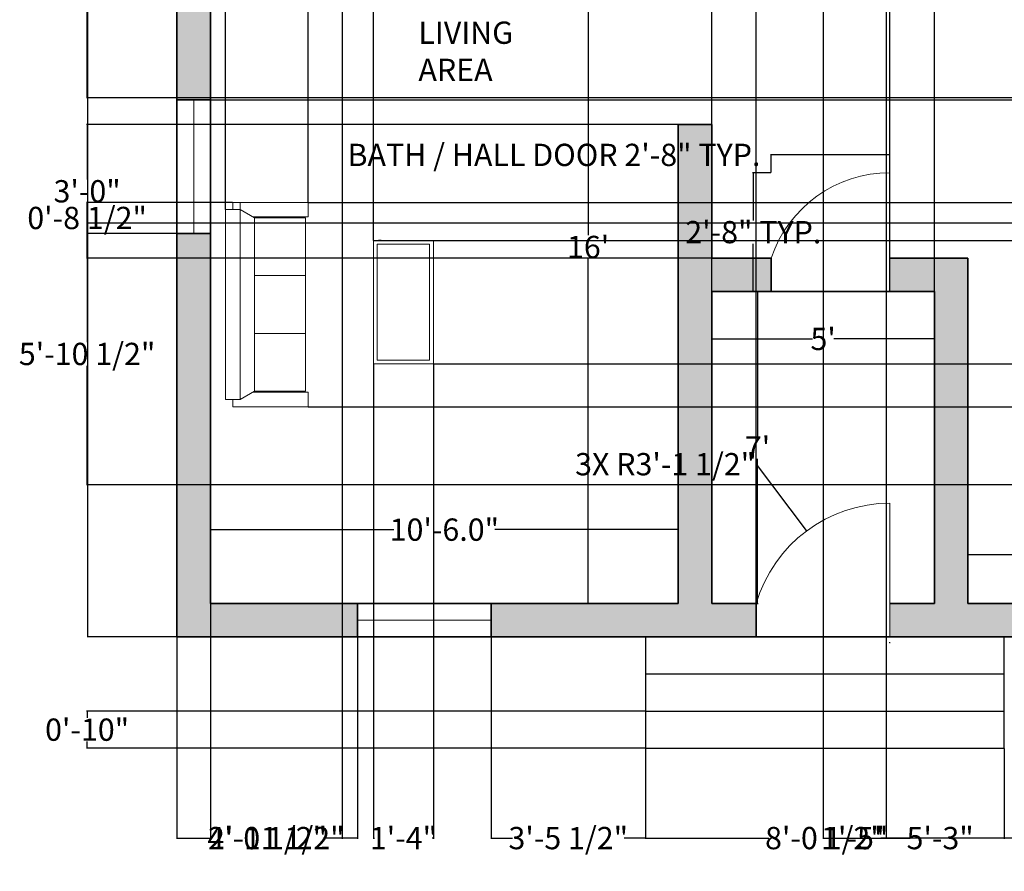
# Model space of a CAD drawing. Units: inches. Extents: x 1174 to 1615, y 3112 to 3628.
# Tile 1 of 6: x 1174 to 1439, y 3112 to 3341. Entities that reach past the tile are written whole.
import ezdxf

# ---------------------------------------------------------------- set-up
doc = ezdxf.new("R2010")
doc.units = ezdxf.units.IN
doc.header["$MEASUREMENT"] = 0
doc.layers.get('0').update_dxf_attribs({"color": 250})
for name, color, linetype, lineweight in [('A-ANNO-DIMS', 2, 'Continuous', 18), ('A-AREA-IDEN', 7, 'Continuous', 25), ('A-DOOR', 3, 'Continuous', 18), ('A-FLOR-STRS', 7, 'Continuous', 25), ('A-FURN', 8, 'Continuous', 13), ('A-GLAZ', 4, 'Continuous', 18), ('A-WALL', 7, 'Continuous', 35)]:
    doc.layers.add(name, color=color, linetype=linetype, lineweight=lineweight)
doc.layers.add('A-WALL-PATT', color=18, linetype='Continuous', lineweight=13, true_color=0x000000)
doc.styles.get("Standard").update_dxf_attribs({"font": 'arial.ttf'})
doc.dimstyles.get("Standard").update_dxf_attribs({"dimtxt": 6, "dimasz": 0.18, "dimexe": 0.18, "dimexo": 0.0625, "dimgap": 0.09, "dimtad": 0, "dimtih": 1, "dimtoh": 1, "dimdec": 1, "dimzin": 0, "dimdsep": 46, "dimlunit": 3, "dimtxsty": 'Standard', "dimcen": 0.09, "dimadec": 0, "dimazin": 0, "dimtfac": 1, "dimtdec": 1, "dimtofl": 0, "dimtmove": 0, "dimatfit": 3, "dimfxl": 1, "dimtolj": 1, "dimtzin": 0, "dimarcsym": 0})

# ---------------------------------------------------------------- blocks, each defined once
blk = doc.blocks.new('*D4')
at = {"layer": 'A-ANNO-DIMS', "color": 0, "lineweight": -2, "transparency": 16777216}
for p, q in [((1216.6, 3595.03), (1192.51, 3595.03)), ((1192.69, 3594.85), (1192.69, 3388.18)), ((1192.69, 3175.21), (1192.69, 3381.87)), ((1216.6, 3175.03), (1192.51, 3175.03))]:
    blk.add_line(p, q, dxfattribs=at)
at = {"layer": 'A-ANNO-DIMS', "color": 0, "transparency": 16777216}
for points in [[(1192.66, 3594.85), (1192.72, 3594.85), (1192.69, 3595.03)], [(1192.66, 3175.21), (1192.72, 3175.21), (1192.69, 3175.03)]]:
    blk.add_solid(points, dxfattribs=at)
at = {"layer": 'Defpoints', "color": 0, "transparency": 16777216}
for p in [(1216.66, 3595.03), (1192.69, 3175.03), (1216.66, 3175.03)]:
    blk.add_point(p, dxfattribs=at)
at = {"layer": 'A-ANNO-DIMS', "color": 0, "transparency": 16777216, "insert": (1192.69, 3385.03), "char_height": 6, "attachment_point": 5}
blk.add_mtext("\\A1;35'", dxfattribs=at)
blk = doc.blocks.new('*D11')
at = {"layer": 'A-ANNO-DIMS', "color": 0, "lineweight": -2, "transparency": 16777216}
for p, q in [((1429.66, 3184.09), (1429.66, 3197.41)), ((1429.84, 3197.23), (1479.05, 3197.23)), ((1555.48, 3197.23), (1506.27, 3197.23)), ((1555.66, 3184.09), (1555.66, 3197.41))]:
    blk.add_line(p, q, dxfattribs=at)
at = {"layer": 'A-ANNO-DIMS', "color": 0, "transparency": 16777216}
for points in [[(1429.84, 3197.26), (1429.84, 3197.2), (1429.66, 3197.23)], [(1555.48, 3197.26), (1555.48, 3197.2), (1555.66, 3197.23)]]:
    blk.add_solid(points, dxfattribs=at)
at = {"layer": 'Defpoints', "color": 0, "transparency": 16777216}
for p in [(1555.66, 3197.23), (1429.66, 3184.03), (1555.66, 3184.03)]:
    blk.add_point(p, dxfattribs=at)
at = {"layer": 'A-ANNO-DIMS', "color": 0, "transparency": 16777216, "insert": (1492.66, 3197.23), "char_height": 6, "attachment_point": 5}
blk.add_mtext('\\A1;10\'-6.0"', dxfattribs=at)
blk = doc.blocks.new('*D13')
at = {"layer": 'A-ANNO-DIMS', "color": 0, "lineweight": -2, "transparency": 16777216}
for p, q in [((1360.73, 3268.03), (1373.17, 3268.03)), ((1372.99, 3267.85), (1372.99, 3229.12)), ((1372.99, 3184.21), (1372.99, 3222.94)), ((1360.73, 3184.03), (1373.17, 3184.03))]:
    blk.add_line(p, q, dxfattribs=at)
at = {"layer": 'A-ANNO-DIMS', "color": 0, "transparency": 16777216}
for points in [[(1372.96, 3267.85), (1373.02, 3267.85), (1372.99, 3268.03)], [(1372.96, 3184.21), (1373.02, 3184.21), (1372.99, 3184.03)]]:
    blk.add_solid(points, dxfattribs=at)
at = {"layer": 'Defpoints', "color": 0, "transparency": 16777216}
for p in [(1360.66, 3268.03), (1372.99, 3268.03), (1360.66, 3184.03)]:
    blk.add_point(p, dxfattribs=at)
at = {"layer": 'A-ANNO-DIMS', "color": 0, "transparency": 16777216, "insert": (1372.99, 3226.03), "char_height": 6, "attachment_point": 5}
blk.add_mtext("\\A1;7'", dxfattribs=at)
blk = doc.blocks.new('*D14')
at = {"layer": 'A-ANNO-DIMS', "color": 0, "lineweight": -2, "transparency": 16777216}
for p, q in [((1360.66, 3267.97), (1360.66, 3255.08)), ((1420.66, 3267.97), (1420.66, 3255.08)), ((1360.84, 3255.26), (1387.81, 3255.26)), ((1420.48, 3255.26), (1393.51, 3255.26))]:
    blk.add_line(p, q, dxfattribs=at)
at = {"layer": 'A-ANNO-DIMS', "color": 0, "transparency": 16777216}
for points in [[(1360.84, 3255.29), (1360.84, 3255.23), (1360.66, 3255.26)], [(1420.48, 3255.29), (1420.48, 3255.23), (1420.66, 3255.26)]]:
    blk.add_solid(points, dxfattribs=at)
at = {"layer": 'Defpoints', "color": 0, "transparency": 16777216}
for p in [(1360.66, 3268.03), (1420.66, 3268.03), (1420.66, 3255.26)]:
    blk.add_point(p, dxfattribs=at)
at = {"layer": 'A-ANNO-DIMS', "color": 0, "transparency": 16777216, "insert": (1390.66, 3255.26), "char_height": 6, "attachment_point": 5}
blk.add_mtext("\\A1;5'", dxfattribs=at)
blk = doc.blocks.new('*D17')
at = {"layer": 'A-ANNO-DIMS', "color": 0, "lineweight": -2, "transparency": 16777216}
for p, q in [((1225.66, 3184.09), (1225.66, 3204.08)), ((1225.84, 3203.9), (1275.05, 3203.9)), ((1351.48, 3203.9), (1302.27, 3203.9)), ((1351.66, 3184.09), (1351.66, 3204.08))]:
    blk.add_line(p, q, dxfattribs=at)
at = {"layer": 'A-ANNO-DIMS', "color": 0, "transparency": 16777216}
for points in [[(1225.84, 3203.93), (1225.84, 3203.87), (1225.66, 3203.9)], [(1351.48, 3203.93), (1351.48, 3203.87), (1351.66, 3203.9)]]:
    blk.add_solid(points, dxfattribs=at)
at = {"layer": 'Defpoints', "color": 0, "transparency": 16777216}
for p in [(1351.66, 3203.9), (1225.66, 3184.03), (1351.66, 3184.03)]:
    blk.add_point(p, dxfattribs=at)
at = {"layer": 'A-ANNO-DIMS', "color": 0, "transparency": 16777216, "insert": (1288.66, 3203.9), "char_height": 6, "attachment_point": 5}
blk.add_mtext('\\A1;10\'-6.0"', dxfattribs=at)
blk = doc.blocks.new('*D18')
at = {"layer": 'A-ANNO-DIMS', "color": 0, "lineweight": -2, "transparency": 16777216}
for p, q in [((1225.73, 3376.03), (1327.55, 3376.03)), ((1327.37, 3375.85), (1327.37, 3283.18)), ((1327.37, 3184.21), (1327.37, 3276.88)), ((1225.73, 3184.03), (1327.55, 3184.03))]:
    blk.add_line(p, q, dxfattribs=at)
at = {"layer": 'A-ANNO-DIMS', "color": 0, "transparency": 16777216}
for points in [[(1327.34, 3375.85), (1327.4, 3375.85), (1327.37, 3376.03)], [(1327.34, 3184.21), (1327.4, 3184.21), (1327.37, 3184.03)]]:
    blk.add_solid(points, dxfattribs=at)
at = {"layer": 'Defpoints', "color": 0, "transparency": 16777216}
for p in [(1225.66, 3376.03), (1225.66, 3184.03), (1327.37, 3184.03)]:
    blk.add_point(p, dxfattribs=at)
at = {"layer": 'A-ANNO-DIMS', "color": 0, "transparency": 16777216, "insert": (1327.37, 3280.03), "char_height": 6, "attachment_point": 5}
blk.add_mtext("\\A1;16'", dxfattribs=at)
blk = doc.blocks.new('DOOR-SWING-36IN')
for p, q in [((-1, 36), (-1, 0)), ((0, 0), (0, 36)), ((0, 0), (-36, 0))]:
    blk.add_line(p, q)
blk.add_arc((0, -1.5), 37.5, 90, 163.7398)
blk = doc.blocks.new('DOOR-SWING-32IN')
for p, q in [((0, 0), (0, -32)), ((0, 0), (32, 0)), ((1, -32), (1, 0))]:
    blk.add_line(p, q)
blk.add_arc((0, 1.76), 33.76, 270, 341.4134)
blk = doc.blocks.new('WINDOW-36IN')
for p, q in [((-4.5, -36), (-4.5, 0)), ((0, 0), (0, -36)), ((4.5, 0), (4.5, -36))]:
    blk.add_line(p, q)
blk = doc.blocks.new('*D38')
at = {"layer": 'A-ANNO-DIMS', "color": 0, "lineweight": -2, "transparency": 16777216}
for p, q in [((1376.66, 3304.83), (1376.48, 3304.83)), ((1376.66, 3300.09), (1376.66, 3305.01)), ((1408.48, 3304.83), (1376.84, 3304.83)), ((1408.66, 3300.09), (1408.66, 3305.01))]:
    blk.add_line(p, q, dxfattribs=at)
at = {"layer": 'A-ANNO-DIMS', "color": 0, "transparency": 16777216}
for points in [[(1376.84, 3304.86), (1376.84, 3304.8), (1376.66, 3304.83)], [(1408.48, 3304.86), (1408.48, 3304.8), (1408.66, 3304.83)]]:
    blk.add_solid(points, dxfattribs=at)
at = {"layer": 'Defpoints', "color": 0, "transparency": 16777216}
for p in [(1376.66, 3304.83), (1376.66, 3300.03), (1408.66, 3300.03)]:
    blk.add_point(p, dxfattribs=at)
at = {"layer": 'A-ANNO-DIMS', "color": 0, "transparency": 16777216, "insert": (1318.18, 3304.83), "char_height": 6, "attachment_point": 5}
blk.add_mtext('\\A1;BATH / HALL DOOR 2\'-8" TYP.', dxfattribs=at)
blk = doc.blocks.new('*D39')
at = {"layer": 'A-ANNO-DIMS', "color": 0, "lineweight": -2, "transparency": 16777216}
for p, q in [((1376.6, 3300.03), (1371.68, 3300.03)), ((1371.86, 3299.85), (1371.86, 3287.18)), ((1371.86, 3268.21), (1371.86, 3280.88)), ((1376.6, 3268.03), (1371.68, 3268.03))]:
    blk.add_line(p, q, dxfattribs=at)
at = {"layer": 'A-ANNO-DIMS', "color": 0, "transparency": 16777216}
for points in [[(1371.83, 3299.85), (1371.89, 3299.85), (1371.86, 3300.03)], [(1371.83, 3268.21), (1371.89, 3268.21), (1371.86, 3268.03)]]:
    blk.add_solid(points, dxfattribs=at)
at = {"layer": 'Defpoints', "color": 0, "transparency": 16777216}
for p in [(1376.66, 3300.03), (1371.86, 3268.03), (1376.66, 3268.03)]:
    blk.add_point(p, dxfattribs=at)
at = {"layer": 'A-ANNO-DIMS', "color": 0, "transparency": 16777216, "insert": (1371.86, 3284.03), "char_height": 6, "attachment_point": 5}
blk.add_mtext('\\A1;2\'-8" TYP.', dxfattribs=at)
blk = doc.blocks.new('*D40')
at = {"layer": 'A-ANNO-DIMS', "color": 0, "lineweight": -2, "transparency": 16777216}
for p, q in [((1342.8, 3144.97), (1342.8, 3120.65)), ((1439.45, 3144.97), (1439.45, 3120.65)), ((1342.98, 3120.83), (1376.07, 3120.83)), ((1439.27, 3120.83), (1406.19, 3120.83))]:
    blk.add_line(p, q, dxfattribs=at)
at = {"layer": 'A-ANNO-DIMS', "color": 0, "transparency": 16777216}
for points in [[(1342.98, 3120.86), (1342.98, 3120.8), (1342.8, 3120.83)], [(1439.27, 3120.86), (1439.27, 3120.8), (1439.45, 3120.83)]]:
    blk.add_solid(points, dxfattribs=at)
at = {"layer": 'Defpoints', "color": 0, "transparency": 16777216}
for p in [(1342.8, 3145.03), (1439.45, 3145.03), (1439.45, 3120.83)]:
    blk.add_point(p, dxfattribs=at)
at = {"layer": 'A-ANNO-DIMS', "color": 0, "transparency": 16777216, "insert": (1391.13, 3120.83), "char_height": 6, "attachment_point": 5}
blk.add_mtext('\\A1;8\'-0 1/2"', dxfattribs=at)
blk = doc.blocks.new('*D42')
at = {"layer": 'A-ANNO-DIMS', "color": 0, "lineweight": -2, "transparency": 16777216}
for p, q in [((1342.74, 3155.03), (1192.28, 3155.03)), ((1192.46, 3154.85), (1192.46, 3153.18)), ((1342.74, 3145.03), (1192.28, 3145.03)), ((1192.46, 3145.21), (1192.46, 3146.88))]:
    blk.add_line(p, q, dxfattribs=at)
at = {"layer": 'A-ANNO-DIMS', "color": 0, "transparency": 16777216}
for points in [[(1192.43, 3154.85), (1192.49, 3154.85), (1192.46, 3155.03)], [(1192.43, 3145.21), (1192.49, 3145.21), (1192.46, 3145.03)]]:
    blk.add_solid(points, dxfattribs=at)
at = {"layer": 'Defpoints', "color": 0, "transparency": 16777216}
for p in [(1192.46, 3155.03), (1342.8, 3155.03), (1342.8, 3145.03)]:
    blk.add_point(p, dxfattribs=at)
at = {"layer": 'A-ANNO-DIMS', "color": 0, "transparency": 16777216, "insert": (1192.46, 3150.03), "char_height": 6, "attachment_point": 5}
blk.add_mtext('\\A1;0\'-10"', dxfattribs=at)
blk = doc.blocks.new('*D43')
at = {"layer": 'A-ANNO-DIMS', "color": 0, "lineweight": -2, "transparency": 16777216}
for p, q in [((1301.25, 3174.97), (1301.25, 3120.65)), ((1342.8, 3174.97), (1342.8, 3120.65)), ((1301.43, 3120.83), (1306.97, 3120.83)), ((1342.62, 3120.83), (1337.08, 3120.83))]:
    blk.add_line(p, q, dxfattribs=at)
at = {"layer": 'A-ANNO-DIMS', "color": 0, "transparency": 16777216}
for points in [[(1301.43, 3120.86), (1301.43, 3120.8), (1301.25, 3120.83)], [(1342.62, 3120.86), (1342.62, 3120.8), (1342.8, 3120.83)]]:
    blk.add_solid(points, dxfattribs=at)
at = {"layer": 'Defpoints', "color": 0, "transparency": 16777216}
for p in [(1301.25, 3175.03), (1342.8, 3175.03), (1342.8, 3120.83)]:
    blk.add_point(p, dxfattribs=at)
at = {"layer": 'A-ANNO-DIMS', "color": 0, "transparency": 16777216, "insert": (1322.03, 3120.83), "char_height": 6, "attachment_point": 5}
blk.add_mtext('\\A1;3\'-5 1/2"', dxfattribs=at)
blk = doc.blocks.new('*D46')
at = {"layer": 'A-ANNO-DIMS', "color": 0, "lineweight": -2, "transparency": 16777216}
for p, q in [((1216.66, 3174.97), (1216.66, 3120.65)), ((1265.25, 3174.97), (1265.25, 3120.65)), ((1216.84, 3120.83), (1225.78, 3120.83)), ((1265.07, 3120.83), (1256.13, 3120.83))]:
    blk.add_line(p, q, dxfattribs=at)
at = {"layer": 'A-ANNO-DIMS', "color": 0, "transparency": 16777216}
for points in [[(1216.84, 3120.86), (1216.84, 3120.8), (1216.66, 3120.83)], [(1265.07, 3120.86), (1265.07, 3120.8), (1265.25, 3120.83)]]:
    blk.add_solid(points, dxfattribs=at)
at = {"layer": 'Defpoints', "color": 0, "transparency": 16777216}
for p in [(1216.66, 3175.03), (1265.25, 3175.03), (1265.25, 3120.83)]:
    blk.add_point(p, dxfattribs=at)
at = {"layer": 'A-ANNO-DIMS', "color": 0, "transparency": 16777216, "insert": (1240.96, 3120.83), "char_height": 6, "attachment_point": 5}
blk.add_mtext('\\A1;4\'-0 1/2"', dxfattribs=at)
blk = doc.blocks.new('*D49')
at = {"layer": 'A-ANNO-DIMS', "color": 0, "lineweight": -2, "transparency": 16777216}
for p, q in [((1225.73, 3376.03), (1589.04, 3376.03)), ((1588.86, 3375.85), (1588.86, 3351.02)), ((1588.86, 3319.81), (1588.86, 3344.64)), ((1225.73, 3319.63), (1589.04, 3319.63))]:
    blk.add_line(p, q, dxfattribs=at)
at = {"layer": 'A-ANNO-DIMS', "color": 0, "transparency": 16777216}
for points in [[(1588.83, 3375.85), (1588.89, 3375.85), (1588.86, 3376.03)], [(1588.83, 3319.81), (1588.89, 3319.81), (1588.86, 3319.63)]]:
    blk.add_solid(points, dxfattribs=at)
at = {"layer": 'Defpoints', "color": 0, "transparency": 16777216}
for p in [(1225.66, 3376.03), (1225.66, 3319.63), (1588.86, 3319.63)]:
    blk.add_point(p, dxfattribs=at)
at = {"layer": 'A-ANNO-DIMS', "color": 0, "transparency": 16777216, "insert": (1588.86, 3347.83), "char_height": 6, "attachment_point": 5}
blk.add_mtext('\\A1;4\'-8 1/2"', dxfattribs=at)
blk = doc.blocks.new('*D52')
at = {"layer": 'A-ANNO-DIMS', "color": 0, "lineweight": -2, "transparency": 16777216}
for p, q in [((1555.6, 3376.03), (1192.28, 3376.03)), ((1192.46, 3375.85), (1192.46, 3351.26)), ((1192.46, 3320.35), (1192.46, 3344.95)), ((1555.6, 3320.17), (1192.28, 3320.17))]:
    blk.add_line(p, q, dxfattribs=at)
at = {"layer": 'A-ANNO-DIMS', "color": 0, "transparency": 16777216}
for points in [[(1192.43, 3375.85), (1192.49, 3375.85), (1192.46, 3376.03)], [(1192.43, 3320.35), (1192.49, 3320.35), (1192.46, 3320.17)]]:
    blk.add_solid(points, dxfattribs=at)
at = {"layer": 'Defpoints', "color": 0, "transparency": 16777216}
for p in [(1555.66, 3376.03), (1192.46, 3320.17), (1555.66, 3320.17)]:
    blk.add_point(p, dxfattribs=at)
at = {"layer": 'A-ANNO-DIMS', "color": 0, "transparency": 16777216, "insert": (1192.46, 3348.1), "char_height": 6, "attachment_point": 5}
blk.add_mtext('\\A1;4\'-8"', dxfattribs=at)
blk = doc.blocks.new('*D53')
at = {"layer": 'A-ANNO-DIMS', "color": 0, "lineweight": -2, "transparency": 16777216}
for p, q in [((1351.6, 3313.03), (1192.28, 3313.03)), ((1192.46, 3312.85), (1192.46, 3298.18)), ((1192.46, 3277.21), (1192.46, 3291.87)), ((1360.6, 3277.03), (1192.28, 3277.03))]:
    blk.add_line(p, q, dxfattribs=at)
at = {"layer": 'A-ANNO-DIMS', "color": 0, "transparency": 16777216}
for points in [[(1192.43, 3312.85), (1192.49, 3312.85), (1192.46, 3313.03)], [(1192.43, 3277.21), (1192.49, 3277.21), (1192.46, 3277.03)]]:
    blk.add_solid(points, dxfattribs=at)
at = {"layer": 'Defpoints', "color": 0, "transparency": 16777216}
for p in [(1351.66, 3313.03), (1192.46, 3277.03), (1360.66, 3277.03)]:
    blk.add_point(p, dxfattribs=at)
at = {"layer": 'A-ANNO-DIMS', "color": 0, "transparency": 16777216, "insert": (1192.46, 3295.03), "char_height": 6, "attachment_point": 5}
blk.add_mtext('\\A1;3\'-0"', dxfattribs=at)
blk = doc.blocks.new('*D57')
at = {"layer": 'A-ANNO-DIMS', "color": 0, "lineweight": -2, "transparency": 16777216}
for p, q in [((1390.66, 3384.97), (1390.66, 3120.65)), ((1407.66, 3384.97), (1407.66, 3120.65)), ((1390.84, 3120.83), (1391.38, 3120.83)), ((1407.48, 3120.83), (1406.95, 3120.83))]:
    blk.add_line(p, q, dxfattribs=at)
at = {"layer": 'A-ANNO-DIMS', "color": 0, "transparency": 16777216}
for points in [[(1390.84, 3120.86), (1390.84, 3120.8), (1390.66, 3120.83)], [(1407.48, 3120.86), (1407.48, 3120.8), (1407.66, 3120.83)]]:
    blk.add_solid(points, dxfattribs=at)
at = {"layer": 'Defpoints', "color": 0, "transparency": 16777216}
for p in [(1390.66, 3385.03), (1407.66, 3385.03), (1407.66, 3120.83)]:
    blk.add_point(p, dxfattribs=at)
at = {"layer": 'A-ANNO-DIMS', "color": 0, "transparency": 16777216, "insert": (1399.16, 3120.83), "char_height": 6, "attachment_point": 5}
blk.add_mtext('\\A1;1\'-5"', dxfattribs=at)
blk = doc.blocks.new('*D58')
at = {"layer": 'A-ANNO-DIMS', "color": 0, "lineweight": -2, "transparency": 16777216}
for p, q in [((1360.66, 3184.09), (1360.66, 3619.41)), ((1360.84, 3619.23), (1372.48, 3619.23)), ((1372.66, 3184.09), (1372.66, 3619.41)), ((1372.66, 3619.23), (1372.84, 3619.23))]:
    blk.add_line(p, q, dxfattribs=at)
at = {"layer": 'A-ANNO-DIMS', "color": 0, "transparency": 16777216}
for points in [[(1360.84, 3619.26), (1360.84, 3619.2), (1360.66, 3619.23)], [(1372.48, 3619.26), (1372.48, 3619.2), (1372.66, 3619.23)]]:
    blk.add_solid(points, dxfattribs=at)
at = {"layer": 'Defpoints', "color": 0, "transparency": 16777216}
for p in [(1372.66, 3619.23), (1360.66, 3184.03), (1372.66, 3184.03)]:
    blk.add_point(p, dxfattribs=at)
at = {"layer": 'A-ANNO-DIMS', "color": 0, "transparency": 16777216, "insert": (1380.63, 3619.23), "char_height": 6, "attachment_point": 5}
blk.add_mtext('\\A1;1\'-0"', dxfattribs=at)
blk = doc.blocks.new('*D59')
at = {"layer": 'A-ANNO-DIMS', "color": 0, "lineweight": -2, "transparency": 16777216}
for p, q in [((1408.66, 3268.09), (1408.66, 3619.41)), ((1408.84, 3619.23), (1420.48, 3619.23)), ((1420.66, 3268.09), (1420.66, 3619.41)), ((1420.66, 3619.23), (1420.84, 3619.23))]:
    blk.add_line(p, q, dxfattribs=at)
at = {"layer": 'A-ANNO-DIMS', "color": 0, "transparency": 16777216}
for points in [[(1408.84, 3619.26), (1408.84, 3619.2), (1408.66, 3619.23)], [(1420.48, 3619.26), (1420.48, 3619.2), (1420.66, 3619.23)]]:
    blk.add_solid(points, dxfattribs=at)
at = {"layer": 'Defpoints', "color": 0, "transparency": 16777216}
for p in [(1420.66, 3619.23), (1408.66, 3268.03), (1420.66, 3268.03)]:
    blk.add_point(p, dxfattribs=at)
at = {"layer": 'A-ANNO-DIMS', "color": 0, "transparency": 16777216, "insert": (1428.63, 3619.23), "char_height": 6, "attachment_point": 5}
blk.add_mtext('\\A1;1\'-0"', dxfattribs=at)
blk = doc.blocks.new('*D60')
at = {"layer": 'A-ANNO-DIMS', "color": 0, "lineweight": -2, "transparency": 16777216}
for p, q in [((1229.72, 3290.15), (1229.72, 3619.41)), ((1229.9, 3619.23), (1230.72, 3619.23)), ((1251.77, 3619.23), (1250.95, 3619.23)), ((1251.95, 3292.11), (1251.95, 3619.41))]:
    blk.add_line(p, q, dxfattribs=at)
at = {"layer": 'A-ANNO-DIMS', "color": 0, "transparency": 16777216}
for points in [[(1229.9, 3619.26), (1229.9, 3619.2), (1229.72, 3619.23)], [(1251.77, 3619.26), (1251.77, 3619.2), (1251.95, 3619.23)]]:
    blk.add_solid(points, dxfattribs=at)
at = {"layer": 'Defpoints', "color": 0, "transparency": 16777216}
for p in [(1251.95, 3619.23), (1251.95, 3292.05), (1229.72, 3290.09)]:
    blk.add_point(p, dxfattribs=at)
at = {"layer": 'A-ANNO-DIMS', "color": 0, "transparency": 16777216, "insert": (1240.84, 3619.23), "char_height": 6, "attachment_point": 5}
blk.add_mtext('\\A1;1\'-10"', dxfattribs=at)
blk = doc.blocks.new('*D61')
at = {"layer": 'A-ANNO-DIMS', "color": 0, "lineweight": -2, "transparency": 16777216}
for p, q in [((1252.014815, 3292.048747), (1589.043286, 3292.048747)), ((1588.863286, 3291.868747), (1588.863286, 3267.616767)), ((1588.863286, 3237.184787), (1588.863286, 3261.436767)), ((1252.014815, 3237.004787), (1589.043286, 3237.004787))]:
    blk.add_line(p, q, dxfattribs=at)
at = {"layer": 'A-ANNO-DIMS', "color": 0, "transparency": 16777216}
for points in [[(1588.833286, 3291.868747), (1588.893286, 3291.868747), (1588.863286, 3292.048747)], [(1588.833286, 3237.184787), (1588.893286, 3237.184787), (1588.863286, 3237.004787)]]:
    blk.add_solid(points, dxfattribs=at)
at = {"layer": 'Defpoints', "color": 0, "transparency": 16777216}
for p in [(1251.952315, 3292.048747), (1251.952315, 3237.004787), (1588.863286, 3237.004787)]:
    blk.add_point(p, dxfattribs=at)
at = {"layer": 'A-ANNO-DIMS', "color": 0, "transparency": 16777216, "insert": (1588.863286, 3264.526767), "char_height": 6, "attachment_point": 5}
blk.add_mtext('\\A1;4\'-7"', dxfattribs=at)
blk = doc.blocks.new('*D62')
at = {"layer": 'A-ANNO-DIMS', "color": 0, "lineweight": -2, "transparency": 16777216}
for p, q in [((1269.57, 3248.47), (1269.57, 3120.65)), ((1285.7, 3248.47), (1285.7, 3120.65)), ((1269.75, 3120.83), (1269.85, 3120.83)), ((1285.52, 3120.83), (1285.42, 3120.83))]:
    blk.add_line(p, q, dxfattribs=at)
at = {"layer": 'A-ANNO-DIMS', "color": 0, "transparency": 16777216}
for points in [[(1269.75, 3120.86), (1269.75, 3120.8), (1269.57, 3120.83)], [(1285.52, 3120.86), (1285.52, 3120.8), (1285.7, 3120.83)]]:
    blk.add_solid(points, dxfattribs=at)
at = {"layer": 'Defpoints', "color": 0, "transparency": 16777216}
for p in [(1269.57, 3248.53), (1285.7, 3248.53), (1285.7, 3120.83)]:
    blk.add_point(p, dxfattribs=at)
at = {"layer": 'A-ANNO-DIMS', "color": 0, "transparency": 16777216, "insert": (1277.64, 3120.83), "char_height": 6, "attachment_point": 5}
blk.add_mtext('\\A1;1\'-4"', dxfattribs=at)
blk = doc.blocks.new('*D63')
at = {"layer": 'A-ANNO-DIMS', "color": 0, "lineweight": -2, "transparency": 16777216}
for p, q in [((1285.77, 3281.75), (1589.04, 3281.75)), ((1588.86, 3281.57), (1588.86, 3268.3)), ((1588.86, 3248.71), (1588.86, 3261.99)), ((1285.77, 3248.53), (1589.04, 3248.53))]:
    blk.add_line(p, q, dxfattribs=at)
at = {"layer": 'A-ANNO-DIMS', "color": 0, "transparency": 16777216}
for points in [[(1588.83, 3281.57), (1588.89, 3281.57), (1588.86, 3281.75)], [(1588.83, 3248.71), (1588.89, 3248.71), (1588.86, 3248.53)]]:
    blk.add_solid(points, dxfattribs=at)
at = {"layer": 'Defpoints', "color": 0, "transparency": 16777216}
for p in [(1285.7, 3281.75), (1285.7, 3248.53), (1588.86, 3248.53)]:
    blk.add_point(p, dxfattribs=at)
at = {"layer": 'A-ANNO-DIMS', "color": 0, "transparency": 16777216, "insert": (1588.86, 3265.14), "char_height": 6, "attachment_point": 5}
blk.add_mtext('\\A1;2\'-9"', dxfattribs=at)
blk = doc.blocks.new('*D64')
at = {"layer": 'A-ANNO-DIMS', "color": 0, "lineweight": -2, "transparency": 16777216}
for p, q in [((1251.95, 3292.11), (1251.95, 3619.41)), ((1252.13, 3619.23), (1269.39, 3619.23)), ((1269.57, 3281.81), (1269.57, 3619.41)), ((1269.57, 3619.23), (1269.75, 3619.23))]:
    blk.add_line(p, q, dxfattribs=at)
at = {"layer": 'A-ANNO-DIMS', "color": 0, "transparency": 16777216}
for points in [[(1252.13, 3619.26), (1252.13, 3619.2), (1251.95, 3619.23)], [(1269.39, 3619.26), (1269.39, 3619.2), (1269.57, 3619.23)]]:
    blk.add_solid(points, dxfattribs=at)
at = {"layer": 'Defpoints', "color": 0, "transparency": 16777216}
for p in [(1269.57, 3619.23), (1251.95, 3292.05), (1269.57, 3281.75)]:
    blk.add_point(p, dxfattribs=at)
at = {"layer": 'A-ANNO-DIMS', "color": 0, "transparency": 16777216, "insert": (1284.52, 3619.23), "char_height": 6, "attachment_point": 5}
blk.add_mtext('\\A1;1\'-5 1/2"', dxfattribs=at)
blk = doc.blocks.new('*D65')
at = {"layer": 'A-ANNO-DIMS', "color": 0, "lineweight": -2, "transparency": 16777216}
for p, q in [((1252.01, 3292.05), (1589.04, 3292.05)), ((1588.86, 3291.87), (1588.86, 3290.09)), ((1588.86, 3281.93), (1588.86, 3283.71)), ((1269.63, 3281.75), (1589.04, 3281.75))]:
    blk.add_line(p, q, dxfattribs=at)
at = {"layer": 'A-ANNO-DIMS', "color": 0, "transparency": 16777216}
for points in [[(1588.83, 3291.87), (1588.89, 3291.87), (1588.86, 3292.05)], [(1588.83, 3281.93), (1588.89, 3281.93), (1588.86, 3281.75)]]:
    blk.add_solid(points, dxfattribs=at)
at = {"layer": 'Defpoints', "color": 0, "transparency": 16777216}
for p in [(1251.95, 3292.05), (1588.86, 3292.05), (1269.57, 3281.75)]:
    blk.add_point(p, dxfattribs=at)
at = {"layer": 'A-ANNO-DIMS', "color": 0, "transparency": 16777216, "insert": (1588.86, 3286.9), "char_height": 6, "attachment_point": 5}
blk.add_mtext('\\A1;0\'-10 1/2"', dxfattribs=at)
blk = doc.blocks.new('*D67')
at = {"layer": 'A-ANNO-DIMS', "color": 0, "lineweight": -2, "transparency": 16777216}
for p, q in [((1475.43, 3286.44), (1192.28, 3286.44)), ((1192.46, 3286.26), (1192.46, 3254.41)), ((1192.46, 3216.17), (1192.46, 3248.02)), ((1475.43, 3215.99), (1192.28, 3215.99))]:
    blk.add_line(p, q, dxfattribs=at)
at = {"layer": 'A-ANNO-DIMS', "color": 0, "transparency": 16777216}
for points in [[(1192.43, 3286.26), (1192.49, 3286.26), (1192.46, 3286.44)], [(1192.43, 3216.17), (1192.49, 3216.17), (1192.46, 3215.99)]]:
    blk.add_solid(points, dxfattribs=at)
at = {"layer": 'Defpoints', "color": 0, "transparency": 16777216}
for p in [(1475.5, 3286.44), (1192.46, 3215.99), (1475.5, 3215.99)]:
    blk.add_point(p, dxfattribs=at)
at = {"layer": 'A-ANNO-DIMS', "color": 0, "transparency": 16777216, "insert": (1192.46, 3251.22), "char_height": 6, "attachment_point": 5}
blk.add_mtext('\\A1;5\'-10 1/2"', dxfattribs=at)
blk = doc.blocks.new('*D69')
at = {"layer": 'A-ANNO-DIMS', "color": 0, "lineweight": -2, "transparency": 16777216}
for p, q in [((1225.66, 3585.97), (1225.66, 3120.65)), ((1261.16, 3585.86), (1261.16, 3120.65)), ((1225.84, 3120.83), (1225.98, 3120.83)), ((1260.98, 3120.83), (1260.85, 3120.83))]:
    blk.add_line(p, q, dxfattribs=at)
at = {"layer": 'A-ANNO-DIMS', "color": 0, "transparency": 16777216}
for points in [[(1225.84, 3120.86), (1225.84, 3120.8), (1225.66, 3120.83)], [(1260.98, 3120.86), (1260.98, 3120.8), (1261.16, 3120.83)]]:
    blk.add_solid(points, dxfattribs=at)
at = {"layer": 'Defpoints', "color": 0, "transparency": 16777216}
for p in [(1225.66, 3586.03), (1261.16, 3585.93), (1261.16, 3120.83)]:
    blk.add_point(p, dxfattribs=at)
at = {"layer": 'A-ANNO-DIMS', "color": 0, "transparency": 16777216, "insert": (1243.41, 3120.83), "char_height": 6, "attachment_point": 5}
blk.add_mtext('\\A1;2\'-11 1/2"', dxfattribs=at)
blk = doc.blocks.new('*D70')
at = {"layer": 'A-ANNO-DIMS', "color": 0, "lineweight": -2, "transparency": 16777216}
for p, q in [((1390.66, 3585.97), (1390.66, 3120.65)), ((1453.68, 3583.03), (1453.68, 3120.65)), ((1390.84, 3120.83), (1414.11, 3120.83)), ((1453.5, 3120.83), (1430.24, 3120.83))]:
    blk.add_line(p, q, dxfattribs=at)
at = {"layer": 'A-ANNO-DIMS', "color": 0, "transparency": 16777216}
for points in [[(1390.84, 3120.86), (1390.84, 3120.8), (1390.66, 3120.83)], [(1453.5, 3120.86), (1453.5, 3120.8), (1453.68, 3120.83)]]:
    blk.add_solid(points, dxfattribs=at)
at = {"layer": 'Defpoints', "color": 0, "transparency": 16777216}
for p in [(1390.66, 3586.03), (1453.68, 3583.1), (1453.68, 3120.83)]:
    blk.add_point(p, dxfattribs=at)
at = {"layer": 'A-ANNO-DIMS', "color": 0, "transparency": 16777216, "insert": (1422.17, 3120.83), "char_height": 6, "attachment_point": 5}
blk.add_mtext('\\A1;5\'-3"', dxfattribs=at)
blk = doc.blocks.new('*D71')
at = {"layer": 'A-ANNO-DIMS', "color": 0, "lineweight": -2, "transparency": 16777216}
for p, q in [((1225.66, 3283.7), (1225.66, 3619.41)), ((1225.84, 3619.23), (1229.54, 3619.23)), ((1229.72, 3290.15), (1229.72, 3619.41)), ((1229.72, 3619.23), (1229.9, 3619.23))]:
    blk.add_line(p, q, dxfattribs=at)
at = {"layer": 'A-ANNO-DIMS', "color": 0, "transparency": 16777216}
for points in [[(1225.84, 3619.26), (1225.84, 3619.2), (1225.66, 3619.23)], [(1229.54, 3619.26), (1229.54, 3619.2), (1229.72, 3619.23)]]:
    blk.add_solid(points, dxfattribs=at)
at = {"layer": 'Defpoints', "color": 0, "transparency": 16777216}
for p in [(1229.72, 3619.23), (1229.72, 3290.09), (1225.66, 3283.63)]:
    blk.add_point(p, dxfattribs=at)
at = {"layer": 'A-ANNO-DIMS', "color": 0, "transparency": 16777216, "insert": (1237.97, 3619.23), "char_height": 6, "attachment_point": 5}
blk.add_mtext('\\A1;0\'-4"', dxfattribs=at)
blk = doc.blocks.new('*D72')
at = {"layer": 'A-ANNO-DIMS', "color": 0, "lineweight": -2, "transparency": 16777216}
for p, q in [((1231.62, 3292.05), (1192.28, 3292.05)), ((1192.46, 3291.87), (1192.46, 3291.03)), ((1225.6, 3283.63), (1192.28, 3283.63)), ((1192.46, 3283.81), (1192.46, 3284.65))]:
    blk.add_line(p, q, dxfattribs=at)
at = {"layer": 'A-ANNO-DIMS', "color": 0, "transparency": 16777216}
for points in [[(1192.43, 3291.87), (1192.49, 3291.87), (1192.46, 3292.05)], [(1192.43, 3283.81), (1192.49, 3283.81), (1192.46, 3283.63)]]:
    blk.add_solid(points, dxfattribs=at)
at = {"layer": 'Defpoints', "color": 0, "transparency": 16777216}
for p in [(1192.46, 3292.05), (1231.68, 3292.05), (1225.66, 3283.63)]:
    blk.add_point(p, dxfattribs=at)
at = {"layer": 'A-ANNO-DIMS', "color": 0, "transparency": 16777216, "insert": (1192.46, 3287.84), "char_height": 6, "attachment_point": 5}
blk.add_mtext('\\A1;0\'-8 1/2"', dxfattribs=at)
blk = doc.blocks.new('*D76')
at = {"layer": 'A-ANNO-DIMS', "color": 0, "lineweight": -2, "transparency": 16777216}
for p, q in [((1372.48, 3221.53), (1372.66, 3221.53)), ((1372.66, 3221.53), (1386.06, 3203.67)), ((1408.57, 3173.53), (1408.75, 3173.53)), ((1408.66, 3173.44), (1408.66, 3173.62))]:
    blk.add_line(p, q, dxfattribs=at)
at = {"layer": 'A-ANNO-DIMS', "color": 0, "transparency": 16777216}
blk.add_solid([(1386.08, 3203.69), (1386.03, 3203.65), (1386.16, 3203.53)], dxfattribs=at)
at = {"layer": 'Defpoints', "color": 0, "transparency": 16777216}
for p in [(1386.16, 3203.53), (1408.66, 3173.53)]:
    blk.add_point(p, dxfattribs=at)
at = {"layer": 'A-ANNO-DIMS', "color": 0, "transparency": 16777216, "insert": (1348.11, 3221.53), "char_height": 6, "attachment_point": 5}
blk.add_mtext('\\A1;3X R3\'-1 1/2"', dxfattribs=at)

msp = doc.modelspace()

# ---------------------------------------------------------------- hatches: boundary and pattern name
at = {"layer": 'A-WALL-PATT'}
h = msp.add_hatch(color=256, dxfattribs=at)
h.dxf.hatch_style = 1
h.paths.add_polyline_path([(1564.66, 3595.03), (1216.66, 3595.03), (1216.66, 3564.55), (1225.66, 3564.55), (1225.66, 3586.03), (1381.66, 3586.03), (1381.66, 3385.03), (1380.66, 3385.03), (1380.66, 3376.03), (1381.66, 3376.03), (1407.66, 3376.03), (1407.66, 3385.03), (1390.66, 3385.03), (1390.66, 3586.03), (1555.66, 3586.03), (1555.66, 3558.83), (1564.66, 3558.83)])
h.paths.add_polyline_path([(1564.66, 3408.64), (1555.66, 3408.64), (1555.66, 3385.03), (1453.66, 3385.03), (1453.66, 3457.03), (1465.66, 3457.03), (1465.66, 3466.03), (1453.66, 3466.03), (1444.66, 3466.03), (1444.66, 3385.03), (1443.66, 3385.03), (1443.66, 3376.03), (1444.66, 3376.03), (1555.66, 3376.03), (1555.66, 3320.17), (1564.66, 3320.17)])
h.paths.add_polyline_path([(1564.66, 3522.83), (1555.66, 3522.83), (1555.66, 3466.03), (1497.66, 3466.03), (1497.66, 3457.03), (1555.66, 3457.03), (1555.66, 3432.64), (1564.66, 3432.64)], flags=17)
h.paths.add_polyline_path([(1344.66, 3385.03), (1336.66, 3385.03), (1336.66, 3466.03), (1269.66, 3466.03), (1269.66, 3457.03), (1327.66, 3457.03), (1327.66, 3385.03), (1225.66, 3385.03), (1225.66, 3413.31), (1216.66, 3413.31), (1216.66, 3319.63), (1225.66, 3319.63), (1225.66, 3376.03), (1344.66, 3376.03)])
h.paths.add_polyline_path([(1237.66, 3466.03), (1225.66, 3466.03), (1225.66, 3528.55), (1216.66, 3528.55), (1216.66, 3437.31), (1225.66, 3437.31), (1225.66, 3457.03), (1237.66, 3457.03)], flags=17)
h.paths.add_polyline_path([(1265.25, 3184.03), (1225.66, 3184.03), (1225.66, 3283.63), (1216.66, 3283.63), (1216.66, 3175.03), (1265.25, 3175.03)])
h.paths.add_polyline_path([(1372.66, 3184.03), (1360.66, 3184.03), (1360.66, 3268.03), (1376.66, 3268.03), (1376.66, 3277.03), (1360.66, 3277.03), (1360.66, 3313.03), (1351.66, 3313.03), (1351.66, 3184.03), (1301.25, 3184.03), (1301.25, 3175.03), (1372.66, 3175.03)])
h.paths.add_polyline_path([(1460.02, 3184.03), (1429.66, 3184.03), (1429.66, 3277.03), (1408.66, 3277.03), (1408.66, 3268.03), (1420.66, 3268.03), (1420.66, 3184.03), (1408.66, 3184.03), (1408.66, 3175.03), (1460.02, 3175.03)])
h.paths.add_polyline_path([(1564.66, 3284.17), (1555.66, 3284.17), (1555.66, 3184.03), (1520.02, 3184.03), (1520.02, 3175.03), (1564.66, 3175.03)])

# ---------------------------------------------------------------- linework, layer by layer
at = {"layer": 'A-DOOR'}
for p, q in [((1408.66, 3300.03), (1408.66, 3268.03)), ((1408.66, 3211.03), (1408.66, 3175.03))]:
    msp.add_line(p, q, dxfattribs=at)
at = {"layer": 'A-FLOR-STRS'}
for p, q in [((1342.8, 3175.03), (1342.8, 3145.03)), ((1439.45, 3145.03), (1439.45, 3175.03)), ((1342.8, 3165.03), (1439.45, 3165.03)), ((1342.8, 3155.03), (1439.45, 3155.03)), ((1342.8, 3145.03), (1439.45, 3145.03))]:
    msp.add_line(p, q, dxfattribs=at)
at = {"layer": 'A-FURN'}
for p, q in [((1231.68, 3292.05), (1251.95, 3292.05)), ((1231.68, 3292.05), (1231.68, 3290.09)), ((1233.65, 3292.05), (1233.65, 3238.97)), ((1251.95, 3288.13), (1251.95, 3292.05)), ((1229.72, 3290.09), (1229.72, 3238.97)), ((1233.65, 3290.09), (1229.72, 3290.09)), ((1233.65, 3290.09), (1237.57, 3287.88)), ((1237.27, 3288.13), (1251.95, 3288.13)), ((1251.3, 3287.88), (1237.57, 3287.88)), ((1251.3, 3272.31), (1237.57, 3272.31)), ((1251.3, 3256.74), (1237.57, 3256.74)), ((1237.57, 3241.17), (1233.65, 3238.97)), ((1237.01, 3240.93), (1251.95, 3240.93)), ((1251.95, 3240.93), (1251.95, 3237)), ((1233.65, 3238.97), (1229.72, 3238.97)), ((1231.68, 3238.97), (1231.68, 3237)), ((1231.68, 3237), (1251.95, 3237))]:
    msp.add_line(p, q, dxfattribs=at)
msp.add_lwpolyline([(1237.57, 3287.88), (1237.57, 3241.17), (1251.3, 3241.17), (1251.3, 3287.88)], dxfattribs=at)
for points in [[(1269.57, 3281.75), (1285.7, 3281.75), (1285.7, 3248.53), (1269.57, 3248.53)], [(1270.57, 3280.75), (1284.7, 3280.75), (1284.7, 3249.53), (1270.57, 3249.53)], [(1271.62, 3281.75), (1270.93, 3281.75), (1270.93, 3281.89), (1271.62, 3281.89)]]:
    msp.add_lwpolyline(points, close=True, dxfattribs=at)
at = {"layer": 'A-WALL'}
for p, q in [((1216.66, 3595.03), (1216.66, 3175.03)), ((1225.66, 3376.03), (1225.66, 3184.03)), ((1216.66, 3319.63), (1225.66, 3319.63)), ((1360.66, 3313.03), (1351.66, 3313.03)), ((1351.66, 3313.03), (1351.66, 3184.03)), ((1360.66, 3277.03), (1360.66, 3313.03)), ((1360.66, 3313.03), (1360.66, 3277.03)), ((1225.66, 3283.63), (1216.66, 3283.63)), ((1360.66, 3277.03), (1376.66, 3277.03)), ((1376.66, 3268.03), (1376.66, 3277.03)), ((1408.66, 3277.03), (1429.66, 3277.03)), ((1429.66, 3277.03), (1429.66, 3184.03)), ((1360.66, 3268.03), (1420.66, 3268.03)), ((1360.66, 3268.03), (1360.66, 3184.03)), ((1420.66, 3268.03), (1408.66, 3268.03)), ((1420.66, 3268.03), (1420.66, 3184.03)), ((1225.66, 3184.03), (1351.66, 3184.03)), ((1265.25, 3184.03), (1265.25, 3175.03)), ((1301.25, 3175.03), (1301.25, 3184.03)), ((1360.66, 3184.03), (1372.66, 3184.03)), ((1372.66, 3175.03), (1372.66, 3184.03)), ((1408.66, 3184.03), (1420.66, 3184.03)), ((1429.66, 3184.03), (1555.66, 3184.03)), ((1216.66, 3175.03), (1564.66, 3175.03)), ((1420.66, 3175.03), (1408.66, 3175.03))]:
    msp.add_line(p, q, dxfattribs=at)

# ---------------------------------------------------------------- block references
at = {"layer": 'A-DOOR', "rotation": 180}
msp.add_blockref('DOOR-SWING-32IN', (1408.66, 3268.03), dxfattribs=at)
at = {"layer": 'A-DOOR'}
msp.add_blockref('DOOR-SWING-36IN', (1408.66, 3175.03), dxfattribs=at)
at = {"layer": 'A-GLAZ'}
for p, rotation in [((1221.16, 3283.63), 180), ((1265.25, 3179.53), 90.00000000000081)]:
    msp.add_blockref('WINDOW-36IN', p, dxfattribs=dict(at, rotation=rotation))

# ---------------------------------------------------------------- texts
at = {"layer": 'A-AREA-IDEN', "insert": (1281.68, 3340.74), "char_height": 6, "attachment_point": 1}
msp.add_mtext_dynamic_manual_height_columns('LIVING \\PAREA', width=72.4132, gutter_width=1, heights=[0], dxfattribs=at)

# ---------------------------------------------------------------- dimensions: what is measured, and where the dimension line sits
at = {"layer": 'A-ANNO-DIMS'}
for base, p1, p2, override, picture, middle in [((1269.57, 3619.23), (1251.95, 3292.05), (1269.57, 3281.75), {"dimdec": 1, "dimlfac": 1, "dimrnd": 0, "dimzin": 1, "dimdsep": 46, "dimlunit": 4, "dimfrac": 2}, '*D64', (1284.52, 3619.23)), ((1229.72, 3619.23), (1225.66, 3283.63), (1229.72, 3290.09), {"dimdec": 1, "dimlfac": 1, "dimrnd": 0, "dimzin": 1, "dimdsep": 46, "dimlunit": 4, "dimfrac": 2}, '*D71', (1237.97, 3619.23)), ((1251.95, 3619.23), (1229.72, 3290.09), (1251.95, 3292.05), {"dimdec": 1, "dimlfac": 1, "dimrnd": 0, "dimzin": 1, "dimdsep": 46, "dimlunit": 4, "dimfrac": 2}, '*D60', (1240.84, 3619.23)), ((1372.66, 3619.23), (1360.66, 3184.03), (1372.66, 3184.03), {"dimdec": 1, "dimlfac": 1, "dimrnd": 0, "dimzin": 1, "dimdsep": 46, "dimlunit": 4, "dimfrac": 2}, '*D58', (1380.63, 3619.23)), ((1420.66, 3619.23), (1408.66, 3268.03), (1420.66, 3268.03), {"dimdec": 1, "dimlfac": 1, "dimrnd": 0, "dimzin": 1, "dimdsep": 46, "dimlunit": 4, "dimfrac": 2}, '*D59', (1428.63, 3619.23)), ((1261.16, 3120.83), (1225.66, 3586.03), (1261.16, 3585.93), {"dimdec": 1, "dimlfac": 1, "dimrnd": 0, "dimzin": 1, "dimdsep": 46, "dimlunit": 4, "dimfrac": 2}, '*D69', (1243.41, 3120.83)), ((1453.68, 3120.83), (1390.66, 3586.03), (1453.68, 3583.1), {"dimdec": 1, "dimlfac": 1, "dimrnd": 0, "dimzin": 1, "dimdsep": 46, "dimlunit": 4, "dimfrac": 2}, '*D70', (1422.17, 3120.83)), ((1407.66, 3120.83), (1390.66, 3385.03), (1407.66, 3385.03), {"dimdec": 1, "dimlfac": 1, "dimrnd": 0, "dimzin": 1, "dimdsep": 46, "dimlunit": 4, "dimfrac": 2}, '*D57', (1399.16, 3120.83)), ((1420.66, 3255.26), (1360.66, 3268.03), (1420.66, 3268.03), {"dimclrd": 0, "dimclre": 0, "dimclrt": 0}, '*D14', (1390.66, 3255.26)), ((1285.7, 3120.83), (1269.57, 3248.53), (1285.7, 3248.53), {"dimdec": 1, "dimlfac": 1, "dimrnd": 0, "dimzin": 1, "dimdsep": 46, "dimlunit": 4, "dimfrac": 2}, '*D62', (1277.64, 3120.83)), ((1351.66, 3203.9), (1225.66, 3184.03), (1351.66, 3184.03), {"dimclrd": 0, "dimclre": 0, "dimclrt": 0}, '*D17', (1288.66, 3203.9)), ((1555.66, 3197.23), (1429.66, 3184.03), (1555.66, 3184.03), {"dimclrd": 0, "dimclre": 0, "dimclrt": 0}, '*D11', (1492.66, 3197.23)), ((1265.25, 3120.83), (1216.66, 3175.03), (1265.25, 3175.03), {"dimdec": 1, "dimlfac": 1, "dimrnd": 0, "dimzin": 1, "dimdsep": 46, "dimlunit": 4, "dimfrac": 2}, '*D46', (1240.96, 3120.83)), ((1342.8038, 3120.8288), (1301.2477, 3175.0288), (1342.8038, 3175.0288), {"dimdec": 1, "dimlfac": 1, "dimrnd": 0, "dimzin": 1, "dimdsep": 46, "dimlunit": 4, "dimfrac": 2}, '*D43', (1322.0257, 3120.8288)), ((1439.4482, 3120.8288), (1342.8038, 3145.0288), (1439.4482, 3145.0288), {"dimdec": 1, "dimlfac": 1, "dimrnd": 0, "dimzin": 1, "dimdsep": 46, "dimlunit": 4, "dimfrac": 2}, '*D40', (1391.126, 3120.8288))]:
    dim = msp.add_linear_dim(base=base, p1=p1, p2=p2, dimstyle='Standard', override=override, dxfattribs=at)
    dim.commit()
    dim.dimension.update_dxf_attribs({"geometry": picture, "text_midpoint": middle})
for base, p1, p2, override, picture, middle in [((1192.69, 3175.03), (1216.66, 3595.03), (1216.66, 3175.03), {"dimclrd": 0, "dimclre": 0, "dimclrt": 0}, '*D4', (1192.69, 3385.03)), ((1192.46, 3320.17), (1555.66, 3376.03), (1555.66, 3320.17), {"dimdec": 1, "dimlfac": 1, "dimrnd": 0, "dimzin": 1, "dimdsep": 46, "dimlunit": 4, "dimfrac": 2}, '*D52', (1192.46, 3348.1)), ((1327.37, 3184.03), (1225.66, 3376.03), (1225.66, 3184.03), {"dimclrd": 0, "dimclre": 0, "dimclrt": 0}, '*D18', (1327.37, 3280.03)), ((1588.86, 3319.63), (1225.66, 3376.03), (1225.66, 3319.63), {"dimdec": 1, "dimlfac": 1, "dimrnd": 0, "dimzin": 1, "dimdsep": 46, "dimlunit": 4, "dimfrac": 2}, '*D49', (1588.86, 3347.83)), ((1192.46, 3277.03), (1351.66, 3313.03), (1360.66, 3277.03), {"dimdec": 1, "dimlfac": 1, "dimrnd": 0, "dimzin": 1, "dimdsep": 46, "dimlunit": 4, "dimfrac": 2}, '*D53', (1192.46, 3295.03)), ((1192.46, 3292.05), (1225.66, 3283.63), (1231.68, 3292.05), {"dimdec": 1, "dimlfac": 1, "dimrnd": 0, "dimzin": 1, "dimdsep": 46, "dimlunit": 4, "dimfrac": 2}, '*D72', (1192.46, 3287.84)), ((1588.86, 3292.05), (1269.57, 3281.75), (1251.95, 3292.05), {"dimdec": 1, "dimlfac": 1, "dimrnd": 0, "dimzin": 1, "dimdsep": 46, "dimlunit": 4, "dimfrac": 2}, '*D65', (1588.86, 3286.9)), ((1588.8633, 3237.0048), (1251.9523, 3292.0487), (1251.9523, 3237.0048), {"dimdec": 1, "dimlfac": 1, "dimrnd": 0, "dimzin": 1, "dimdsep": 46, "dimlunit": 4, "dimfrac": 2}, '*D61', (1588.8633, 3264.5268)), ((1192.4633, 3215.9918), (1475.4958, 3286.439), (1475.4958, 3215.9918), {"dimdec": 1, "dimlfac": 1, "dimrnd": 0, "dimzin": 1, "dimdsep": 46, "dimlunit": 4, "dimfrac": 2}, '*D67', (1192.4633, 3251.2154)), ((1588.86, 3248.53), (1285.7, 3281.75), (1285.7, 3248.53), {"dimdec": 1, "dimlfac": 1, "dimrnd": 0, "dimzin": 1, "dimdsep": 46, "dimlunit": 4, "dimfrac": 2}, '*D63', (1588.86, 3265.14)), ((1372.99, 3268.03), (1360.66, 3184.03), (1360.66, 3268.03), {"dimclrd": 0, "dimclre": 0, "dimclrt": 0}, '*D13', (1372.99, 3226.03)), ((1192.46, 3155.03), (1342.8, 3145.03), (1342.8, 3155.03), {"dimdec": 1, "dimlfac": 1, "dimrnd": 0, "dimzin": 1, "dimdsep": 46, "dimlunit": 4, "dimfrac": 2}, '*D42', (1192.46, 3150.03))]:
    dim = msp.add_linear_dim(base=base, p1=p1, p2=p2, angle=90, dimstyle='Standard', override=override, dxfattribs=at)
    dim.commit()
    dim.dimension.update_dxf_attribs({"geometry": picture, "text_midpoint": middle})
for base, p1, p2, angle, text, picture, middle in [((1376.66, 3304.83), (1408.66, 3300.03), (1376.66, 3300.03), 180, 'BATH / HALL DOOR <> TYP.', '*D38', (1318.18, 3304.83)), ((1371.86, 3268.03), (1376.66, 3300.03), (1376.66, 3268.03), 270, '<> TYP.', '*D39', (1371.86, 3284.03))]:
    dim = msp.add_linear_dim(base=base, p1=p1, p2=p2, angle=angle, text=text, dimstyle='Standard', override={"dimdec": 1, "dimlfac": 1, "dimrnd": 0, "dimzin": 1, "dimdsep": 46, "dimlunit": 4, "dimfrac": 2}, dxfattribs=at)
    dim.commit()
    dim.dimension.update_dxf_attribs({"geometry": picture, "text_midpoint": middle})
dim = msp.add_radius_dim(center=(1408.66, 3173.53), mpoint=(1386.16, 3203.53), text='3X <>', dimstyle='Standard', override={"dimdec": 1, "dimlfac": 1, "dimrnd": 0, "dimzin": 1, "dimdsep": 46, "dimlunit": 4, "dimfrac": 2}, dxfattribs=at)
dim.commit()
dim.dimension.update_dxf_attribs({"geometry": '*D76', "text_midpoint": (1348.11, 3221.53), "dimtype": 164})

doc.saveas('drawing.dxf')
